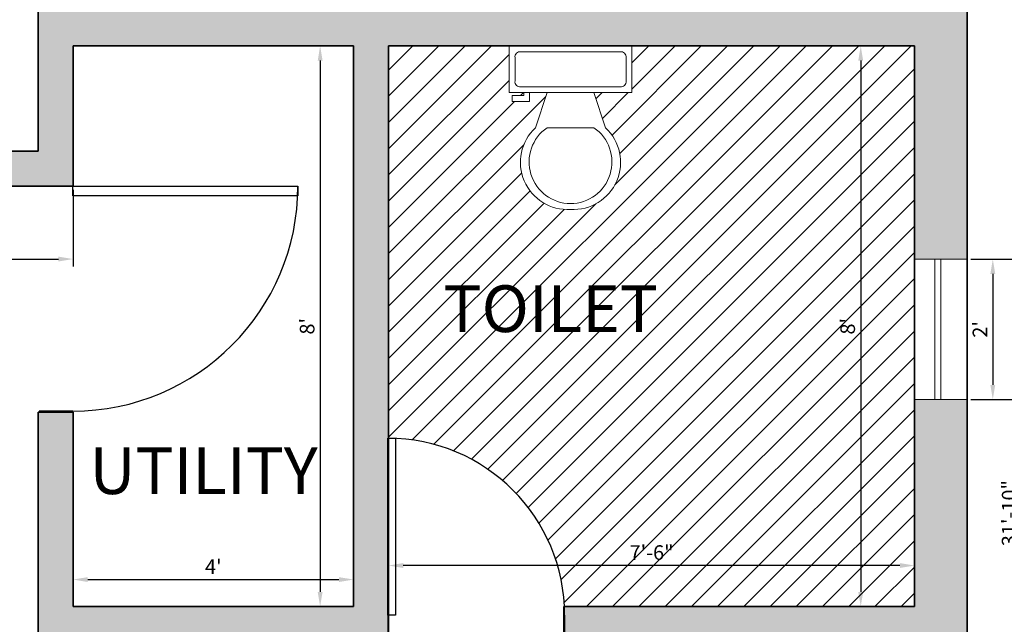
# Model space of a CAD drawing. Units: inches. Extents: x 2901 to 5923, y 918 to 2827.
# Tile 12 of 16: x 4730 to 4898, y 1420 to 1524. Entities that reach past the tile are written whole.
import ezdxf

# ---------------------------------------------------------------- set-up
doc = ezdxf.new("R2010")
doc.units = ezdxf.units.IN
for name, color, linetype, lineweight in [('A-ANNO-DIMS', 2, 'Continuous', 18), ('A-AREA-IDEN', 7, 'Continuous', 25), ('A-FLOR-FIXT', 9, 'Continuous', 18), ('A-FLOR-PATT', 252, 'Continuous', 13), ('A-GLAZ', 4, 'Continuous', 18), ('A-WALL-PATT', 7, 'Continuous', 13), ('doors', 240, 'Continuous', 25), ('walls', 7, 'Continuous', 35)]:
    doc.layers.add(name, color=color, linetype=linetype, lineweight=lineweight)
doc.styles.get("Standard").update_dxf_attribs({"font": 'arial.ttf'})
doc.dimstyles.new('Copy of ISO-25', dxfattribs={"dimtxt": 2.5, "dimasz": 2.5, "dimexe": 1.25, "dimexo": 0.625, "dimtad": 1, "dimdec": 1, "dimlunit": 4, "dimtxsty": 'Standard', "dimcen": 2.5, "dimadec": 0, "dimazin": 0, "dimtfac": 1, "dimtdec": 1, "dimtmove": 0, "dimatfit": 3, "dimfxl": 1, "dimarcsym": 0})

# ---------------------------------------------------------------- blocks, each defined once
blk = doc.blocks.new('*U4')
for p, q in [((-40, 0), (-40, 6)), ((0, 0), (0, 6))]:
    blk.add_line(p, q)
blk.add_lwpolyline([(0, 0), (0, -40), (-1.75, -40), (-1.75, 0)], close=True)
blk.add_arc((0, 0), 40, 180, 270)
blk = doc.blocks.new('*U2')
for p, q in [((0, 0), (0, -6)), ((40, 0), (40, -6))]:
    blk.add_line(p, q)
blk.add_lwpolyline([(0, 0), (0, 40), (1.75, 40), (1.75, 0)], close=True)
blk.add_arc((0, 0), 40, 0, 90)
blk = doc.blocks.new('*U20')
for p, q in [((241.3, -152.4), (241.3, -50.8)), ((-203.2, -215.9), (-203.2, -203.2)), ((-177.8, -203.2), (-177.8, -241.3)), ((-101.6, -203.2), (-152.4, -355.6)), ((101.6, -203.2), (152.4, -355.6)), ((-254, -215.9), (-203.2, -215.9)), ((-254, -241.3), (-254, -215.9)), ((-177.8, -241.3), (-254, -241.3)), ((101.6, -355.6), (-101.6, -355.6))]:
    blk.add_line(p, q)
blk.add_lwpolyline([(266.7, -203.2), (266.7, 0), (-266.7, 0), (-266.7, -203.2)], close=True)
for points in [[(215.9, -25.4), (-215.9, -25.4)], [(-241.3, -50.8), (-241.3, -152.4)], [(-215.9, -177.8), (215.9, -177.8)]]:
    blk.add_lwpolyline(points)
for centre, radius, start, end in [((-219.075, -47.625), 22.45064, 81.8699, 188.1301), ((219.075, -47.625), 22.45064, 351.8699, 98.1301), ((-219.075, -155.575), 22.45064, 171.869898, 278.1301), ((219.075, -155.575), 22.45064, 261.8699, 8.1301), ((-12.12088, -505.93752), 205.61935, 133.01722, 273.38), ((0.94996, -504.77674), 181.02486, 124.50543, 269.7), ((-0.94742, -504.77674), 181.02486, 270.3, 55.4946), ((12.12342, -505.93752), 205.61935, 266.62, 46.9828)]:
    blk.add_arc(centre, radius, start, end)
blk = doc.blocks.new('*D35')
at = {"layer": 'A-ANNO-DIMS', "color": 0, "lineweight": -2, "transparency": 16777216}
for p, q in [((4892.69, 1630.4), (4902.74, 1630.4)), ((4901.49, 1250.9), (4901.49, 1627.9)), ((4892.69, 1248.4), (4902.74, 1248.4))]:
    blk.add_line(p, q, dxfattribs=at)
at = {"layer": 'A-ANNO-DIMS', "color": 0, "transparency": 16777216}
for points in [[(4901.07, 1627.9), (4901.91, 1627.9), (4901.49, 1630.4)], [(4901.07, 1250.9), (4901.91, 1250.9), (4901.49, 1248.4)]]:
    blk.add_solid(points, dxfattribs=at)
at = {"layer": 'Defpoints', "color": 0, "transparency": 16777216}
for p in [(4892.07, 1630.4), (4901.49, 1630.4), (4892.07, 1248.4)]:
    blk.add_point(p, dxfattribs=at)
at = {"layer": 'A-ANNO-DIMS', "color": 0, "transparency": 16777216, "insert": (4899.59, 1439.4), "char_height": 2.5, "attachment_point": 5, "rotation": 90}
blk.add_mtext('31\'-10"', dxfattribs=at)
blk = doc.blocks.new('*D44')
at = {"layer": 'A-ANNO-DIMS', "color": 0, "lineweight": -2, "transparency": 16777216}
for p, q in [((4882.44, 1519.4), (4872.62, 1519.4)), ((4873.87, 1516.9), (4873.87, 1425.9)), ((4882.44, 1423.4), (4872.62, 1423.4))]:
    blk.add_line(p, q, dxfattribs=at)
at = {"layer": 'A-ANNO-DIMS', "color": 0, "transparency": 16777216}
for points in [[(4873.45, 1516.9), (4874.28, 1516.9), (4873.87, 1519.4)], [(4873.45, 1425.9), (4874.28, 1425.9), (4873.87, 1423.4)]]:
    blk.add_solid(points, dxfattribs=at)
at = {"layer": 'Defpoints', "color": 0, "transparency": 16777216}
for p in [(4883.07, 1519.4), (4873.87, 1423.4), (4883.07, 1423.4)]:
    blk.add_point(p, dxfattribs=at)
at = {"layer": 'A-ANNO-DIMS', "color": 0, "transparency": 16777216, "insert": (4871.96, 1471.4), "char_height": 2.5, "attachment_point": 5, "rotation": 90}
blk.add_mtext("8'", dxfattribs=at)
blk = doc.blocks.new('*D45')
at = {"layer": 'A-ANNO-DIMS', "color": 0, "lineweight": -2, "transparency": 16777216}
for p, q in [((4793.07, 1424.02), (4793.07, 1431.68)), ((4883.07, 1424.02), (4883.07, 1431.68)), ((4880.57, 1430.43), (4795.57, 1430.43))]:
    blk.add_line(p, q, dxfattribs=at)
at = {"layer": 'A-ANNO-DIMS', "color": 0, "transparency": 16777216}
for points in [[(4795.57, 1430.85), (4795.57, 1430.01), (4793.07, 1430.43)], [(4880.57, 1430.85), (4880.57, 1430.01), (4883.07, 1430.43)]]:
    blk.add_solid(points, dxfattribs=at)
at = {"layer": 'Defpoints', "color": 0, "transparency": 16777216}
for p in [(4793.07, 1430.43), (4793.07, 1423.4), (4883.07, 1423.4)]:
    blk.add_point(p, dxfattribs=at)
at = {"layer": 'A-ANNO-DIMS', "color": 0, "transparency": 16777216, "insert": (4838.07, 1432.33), "char_height": 2.5, "attachment_point": 5}
blk.add_mtext('7\'-6"', dxfattribs=at)
blk = doc.blocks.new('*D46')
at = {"layer": 'A-ANNO-DIMS', "color": 0, "lineweight": -2, "transparency": 16777216}
for p, q in [((4739.07, 1424.02), (4739.07, 1429.28)), ((4787.07, 1424.02), (4787.07, 1429.28)), ((4741.57, 1428.03), (4784.57, 1428.03))]:
    blk.add_line(p, q, dxfattribs=at)
at = {"layer": 'A-ANNO-DIMS', "color": 0, "transparency": 16777216}
for points in [[(4741.57, 1428.44), (4741.57, 1427.61), (4739.07, 1428.03)], [(4784.57, 1428.44), (4784.57, 1427.61), (4787.07, 1428.03)]]:
    blk.add_solid(points, dxfattribs=at)
at = {"layer": 'Defpoints', "color": 0, "transparency": 16777216}
for p in [(4787.07, 1428.03), (4739.07, 1423.4), (4787.07, 1423.4)]:
    blk.add_point(p, dxfattribs=at)
at = {"layer": 'A-ANNO-DIMS', "color": 0, "transparency": 16777216, "insert": (4763.07, 1429.9), "char_height": 2.5, "attachment_point": 5}
blk.add_mtext("4'", dxfattribs=at)
blk = doc.blocks.new('*D47')
at = {"layer": 'A-ANNO-DIMS', "color": 0, "lineweight": -2, "transparency": 16777216}
for p, q in [((4786.44, 1519.4), (4780.1, 1519.4)), ((4781.35, 1516.9), (4781.35, 1425.9)), ((4786.44, 1423.4), (4780.1, 1423.4))]:
    blk.add_line(p, q, dxfattribs=at)
at = {"layer": 'A-ANNO-DIMS', "color": 0, "transparency": 16777216}
for points in [[(4780.94, 1516.9), (4781.77, 1516.9), (4781.35, 1519.4)], [(4780.94, 1425.9), (4781.77, 1425.9), (4781.35, 1423.4)]]:
    blk.add_solid(points, dxfattribs=at)
at = {"layer": 'Defpoints', "color": 0, "transparency": 16777216}
for p in [(4787.07, 1519.4), (4781.35, 1423.4), (4787.07, 1423.4)]:
    blk.add_point(p, dxfattribs=at)
at = {"layer": 'A-ANNO-DIMS', "color": 0, "transparency": 16777216, "insert": (4779.45, 1471.4), "char_height": 2.5, "attachment_point": 5, "rotation": 90}
blk.add_mtext("8'", dxfattribs=at)
blk = doc.blocks.new('*D56')
at = {"layer": 'A-ANNO-DIMS', "color": 0, "lineweight": -2, "transparency": 16777216}
for p, q in [((4589.07, 1494.77), (4589.07, 1481.66)), ((4739.07, 1494.77), (4739.07, 1481.66)), ((4591.57, 1482.91), (4736.57, 1482.91))]:
    blk.add_line(p, q, dxfattribs=at)
at = {"layer": 'A-ANNO-DIMS', "color": 0, "transparency": 16777216}
for points in [[(4591.57, 1483.32), (4591.57, 1482.49), (4589.07, 1482.91)], [(4736.57, 1483.32), (4736.57, 1482.49), (4739.07, 1482.91)]]:
    blk.add_solid(points, dxfattribs=at)
at = {"layer": 'Defpoints', "color": 0, "transparency": 16777216}
for p in [(4589.07, 1495.4), (4739.07, 1495.4), (4739.07, 1482.91)]:
    blk.add_point(p, dxfattribs=at)
at = {"layer": 'A-ANNO-DIMS', "color": 0, "transparency": 16777216, "insert": (4664.07, 1484.81), "char_height": 2.5, "attachment_point": 5}
blk.add_mtext('12\'-6"', dxfattribs=at)
blk = doc.blocks.new('*D69')
at = {"layer": 'A-ANNO-DIMS', "color": 0, "lineweight": -2, "transparency": 16777216}
for p, q in [((4892.69, 1482.87), (4897.72, 1482.87)), ((4896.47, 1480.37), (4896.47, 1461.37)), ((4892.69, 1458.87), (4897.72, 1458.87))]:
    blk.add_line(p, q, dxfattribs=at)
at = {"layer": 'A-ANNO-DIMS', "color": 0, "transparency": 16777216}
for points in [[(4896.05, 1480.37), (4896.89, 1480.37), (4896.47, 1482.87)], [(4896.05, 1461.37), (4896.89, 1461.37), (4896.47, 1458.87)]]:
    blk.add_solid(points, dxfattribs=at)
at = {"layer": 'Defpoints', "color": 0, "transparency": 16777216}
for p in [(4892.07, 1482.87), (4892.07, 1458.87), (4896.47, 1458.87)]:
    blk.add_point(p, dxfattribs=at)
at = {"layer": 'A-ANNO-DIMS', "color": 0, "transparency": 16777216, "insert": (4894.59, 1470.87), "char_height": 2.5, "attachment_point": 5, "rotation": 90}
blk.add_mtext("2'", dxfattribs=at)
blk = doc.blocks.new('*D89')
at = {"layer": 'A-ANNO-DIMS', "color": 0, "lineweight": -2, "transparency": 16777216}
for p, q in [((4892.69, 1630.4), (5055.73, 1630.4)), ((5054.48, 989.9), (5054.48, 1627.9)), ((4709.69, 987.4), (5055.73, 987.4))]:
    blk.add_line(p, q, dxfattribs=at)
at = {"layer": 'A-ANNO-DIMS', "color": 0, "transparency": 16777216}
for points in [[(5054.06, 1627.9), (5054.9, 1627.9), (5054.48, 1630.4)], [(5054.06, 989.9), (5054.9, 989.9), (5054.48, 987.4)]]:
    blk.add_solid(points, dxfattribs=at)
at = {"layer": 'Defpoints', "color": 0, "transparency": 16777216}
for p in [(4892.07, 1630.4), (5054.48, 1630.4), (4709.07, 987.4)]:
    blk.add_point(p, dxfattribs=at)
at = {"layer": 'A-ANNO-DIMS', "color": 0, "transparency": 16777216, "insert": (5052.58, 1308.9), "char_height": 2.5, "attachment_point": 5, "rotation": 90}
blk.add_mtext('53\'-7"', dxfattribs=at)
blk = doc.blocks.new('*D96')
at = {"layer": 'A-ANNO-DIMS', "color": 0, "lineweight": -2, "transparency": 16777216}
for p, q in [((4892.69, 1630.4), (5055.73, 1630.4)), ((5054.48, 1627.9), (5054.48, 1485.37)), ((4892.69, 1482.87), (5055.73, 1482.87))]:
    blk.add_line(p, q, dxfattribs=at)
at = {"layer": 'A-ANNO-DIMS', "color": 0, "transparency": 16777216}
for points in [[(5054.06, 1627.9), (5054.9, 1627.9), (5054.48, 1630.4)], [(5054.06, 1485.37), (5054.9, 1485.37), (5054.48, 1482.87)]]:
    blk.add_solid(points, dxfattribs=at)
at = {"layer": 'Defpoints', "color": 0, "transparency": 16777216}
for p in [(4892.07, 1630.4), (4892.07, 1482.87), (5054.48, 1482.87)]:
    blk.add_point(p, dxfattribs=at)
at = {"layer": 'A-ANNO-DIMS', "color": 0, "transparency": 16777216, "insert": (5052.56, 1556.63), "char_height": 2.5, "attachment_point": 5, "rotation": 90}
blk.add_mtext('12\'-3 1/2"', dxfattribs=at)
blk = doc.blocks.new('*D97')
at = {"layer": 'A-ANNO-DIMS', "color": 0, "lineweight": -2, "transparency": 16777216}
for p, q in [((4892.69, 1458.87), (5055.73, 1458.87)), ((5054.48, 1456.37), (5054.48, 1365.81)), ((4892.69, 1363.31), (5055.73, 1363.31))]:
    blk.add_line(p, q, dxfattribs=at)
at = {"layer": 'A-ANNO-DIMS', "color": 0, "transparency": 16777216}
for points in [[(5054.06, 1456.37), (5054.9, 1456.37), (5054.48, 1458.87)], [(5054.06, 1365.81), (5054.9, 1365.81), (5054.48, 1363.31)]]:
    blk.add_solid(points, dxfattribs=at)
at = {"layer": 'Defpoints', "color": 0, "transparency": 16777216}
for p in [(4892.07, 1458.87), (4892.07, 1363.31), (5054.48, 1363.31)]:
    blk.add_point(p, dxfattribs=at)
at = {"layer": 'A-ANNO-DIMS', "color": 0, "transparency": 16777216, "insert": (5052.56, 1411.09), "char_height": 2.5, "attachment_point": 5, "rotation": 90}
blk.add_mtext('7\'-11 1/2"', dxfattribs=at)

msp = doc.modelspace()

# ---------------------------------------------------------------- hatches: boundary and pattern name
at = {"layer": 'A-FLOR-PATT'}
h = msp.add_hatch(dxfattribs=at)
h.set_pattern_fill('ANSI32', color=256)
h.paths.add_polyline_path([(4883.07, 1621.4), (4739.07, 1621.4), (4739.07, 1564.39, -0.396616), (4774.43, 1529.97), (4774.46, 1529.97), (4774.46, 1528.4), (4883.07, 1528.4)])
h.paths.add_polyline_path([(4733.07, 1143.4), (4685.07, 1143.4), (4685.07, 1147.03), (4684.01, 1147.03), (4684.01, 1171.22, 0.413071), (4660.87, 1146.06, 0.412532), (4638.11, 1170.77), (4638.11, 1146.97), (4637.07, 1143.4), (4589.07, 1143.4), (4589.07, 1029.4), (4733.07, 1029.4)])
h.paths.add_polyline_path([(4620.35, 1086.26, -0.333335), (4622.56, 1084.04), (4622.56, 1084.04), (4712.62, 1084.04, -0.333335), (4714.84, 1086.26), (4718.53, 1086.26, -0.376086), (4721.48, 1084.04), (4721.48, 1062.64), (4721.48, 1041.23, -0.333387), (4718.96, 1039.01), (4714.84, 1039.01, -0.333335), (4712.62, 1041.23), (4712.62, 1041.23), (4622.56, 1041.23, -0.333335), (4620.35, 1039.01), (4616.66, 1039.01, -0.376086), (4613.71, 1041.23), (4613.71, 1062.63), (4613.71, 1084.04, -0.333387), (4616.23, 1086.26)], flags=16)
h.paths.add_polyline_path([(4638.8, 1084.04), (4643.23, 1078.14), (4678.67, 1078.14), (4687.53, 1084.04), (4687.53, 1071.49), (4718.53, 1067.06), (4718.53, 1062.64), (4718.53, 1058.21), (4687.53, 1053.78), (4687.53, 1041.23), (4678.67, 1047.13), (4643.23, 1047.13), (4638.8, 1041.23), (4638.8, 1062.63)], flags=0)
h = msp.add_hatch(dxfattribs=at)
h.set_pattern_fill('ANSI31', color=256)
h.paths.add_polyline_path([(4883.07, 1519.4), (4834.7, 1519.4), (4834.7, 1511.4), (4828.2, 1511.4), (4830.2, 1505.4, -0.702571), (4824.2, 1491.4, -0.702562), (4818.2, 1505.4), (4820.2, 1511.4), (4817.2, 1511.4), (4817.2, 1509.9), (4814.2, 1509.9), (4814.2, 1510.9), (4816.2, 1510.9), (4816.2, 1511.4), (4813.7, 1511.4), (4813.7, 1519.4), (4793.07, 1519.4), (4793.07, 1452.23), (4794.23, 1452.23), (4794.23, 1452.2, -0.387553), (4823.16, 1423.4), (4883.07, 1423.4)])
at = {"layer": 'A-WALL-PATT'}
h = msp.add_hatch(color=256, dxfattribs=at)
h.dxf.hatch_style = 1
h.paths.add_polyline_path([(4439.07, 1447.4), (4583.07, 1447.4), (4583.07, 1340.4), (4589.07, 1340.4), (4589.07, 1453.4), (4589.07, 1455.39), (4583.07, 1455.39), (4583.07, 1453.4), (4439.07, 1453.4), (4439.07, 1501.84), (4430.07, 1501.84), (4430.07, 1399.4), (4439.07, 1399.4)])
h.paths.add_polyline_path([(4439.07, 1621.4), (4487.07, 1621.4), (4487.07, 1630.4), (4430.07, 1630.4), (4430.07, 1561.84), (4439.07, 1561.84)])
h.paths.add_polyline_path([(4630.61, 1630.4), (4535.07, 1630.4), (4535.07, 1621.4), (4583.07, 1621.4), (4583.07, 1495.4), (4589.07, 1495.4), (4637.07, 1495.4), (4637.07, 1501.4), (4589.07, 1501.4), (4589.07, 1621.4), (4630.61, 1621.4)])
h.paths.add_polyline_path([(4892.07, 1630.4), (4690.61, 1630.4), (4690.61, 1621.4), (4733.07, 1621.4), (4733.07, 1564.4), (4739.07, 1564.4), (4739.07, 1621.4), (4883.07, 1621.4), (4883.07, 1528.4), (4739.07, 1528.4), (4733.07, 1528.4), (4733.07, 1501.4), (4685.07, 1501.4), (4685.07, 1495.4), (4739.07, 1495.4), (4739.07, 1519.4), (4787.07, 1519.4), (4787.07, 1423.4), (4739.07, 1423.4), (4739.07, 1456.67), (4733.07, 1456.67), (4733.07, 1340.4), (4739.07, 1340.4), (4739.07, 1417.4), (4787.07, 1417.4), (4793.07, 1417.4), (4793.07, 1423.4), (4793.07, 1519.4), (4883.07, 1519.4), (4883.07, 1482.87), (4892.07, 1482.87)])
h.paths.add_polyline_path([(4892.07, 1458.87), (4883.07, 1458.87), (4883.07, 1423.4), (4823.07, 1423.4), (4823.07, 1417.4), (4883.07, 1417.4), (4883.07, 1363.31), (4892.07, 1363.31)], flags=17)
h.paths.add_polyline_path([(4892.07, 1303.31), (4883.07, 1303.31), (4883.07, 1255.4), (4739.07, 1255.4), (4739.07, 1304.4), (4733.07, 1304.4), (4733.07, 1303.4), (4733.07, 1297.4), (4733.07, 1255.4), (4733.07, 1248.4), (4811.07, 1248.4), (4811.07, 1212.16), (4820.07, 1212.16), (4820.07, 1248.4), (4892.07, 1248.4)])
h.paths.add_polyline_path([(4820.07, 1182.16), (4811.07, 1182.16), (4811.07, 1152.4), (4685.07, 1152.4), (4685.07, 1147.03), (4685.07, 1143.4), (4733.07, 1143.4), (4811.07, 1143.4), (4814.07, 1143.4), (4820.07, 1143.4)])
h.paths.add_polyline_path([(4637.07, 1152.4), (4589.07, 1152.4), (4589.07, 1153.4), (4583.86, 1153.4), (4583.07, 1153.4), (4583.07, 1152.4), (4511.07, 1152.4), (4511.07, 1182.16), (4502.07, 1182.16), (4502.07, 1143.4), (4568.07, 1143.4), (4583.07, 1143.4), (4583.07, 1023.4), (4739.07, 1023.4), (4739.07, 1143.4), (4733.07, 1143.4), (4733.07, 1029.4), (4589.07, 1029.4), (4589.07, 1143.4), (4637.07, 1143.4), (4637.07, 1146.97)])
h.paths.add_polyline_path([(4511.07, 1246.4), (4583.07, 1246.4), (4583.07, 1188.4), (4589.07, 1188.4), (4589.07, 1246.4), (4589.07, 1248.4), (4589.07, 1255.4), (4589.07, 1297.4), (4697.07, 1297.4), (4697.07, 1303.4), (4589.07, 1303.4), (4589.07, 1304.4), (4583.07, 1304.4), (4583.07, 1255.4), (4439.07, 1255.4), (4439.07, 1261.4), (4439.07, 1351.4), (4430.07, 1351.4), (4430.07, 1252.4), (4430.07, 1246.4), (4439.07, 1246.4), (4487.07, 1246.4), (4502.07, 1246.4), (4502.07, 1212.16), (4511.07, 1212.16)])

# ---------------------------------------------------------------- linework, layer by layer
at = {"layer": 'A-GLAZ'}
for p, q in [((4883.07, 1482.87), (4892.07, 1482.87)), ((4886.57, 1482.87), (4886.57, 1458.87)), ((4887.57, 1482.87), (4887.57, 1458.87)), ((4892.07, 1482.87), (4892.07, 1458.87)), ((4892.07, 1458.87), (4883.07, 1458.87))]:
    msp.add_line(p, q, dxfattribs=at)
at = {"layer": 'walls'}
for p, q in [((4892.07, 1630.4), (4892.07, 1248.4)), ((4733.07, 1528.4), (4733.07, 1501.4)), ((4739.07, 1519.4), (4787.07, 1519.4)), ((4787.07, 1519.4), (4739.07, 1519.4)), ((4739.07, 1519.4), (4739.07, 1495.4)), ((4787.07, 1519.4), (4787.07, 1423.4)), ((4883.07, 1519.4), (4793.07, 1519.4)), ((4883.07, 1519.4), (4793.07, 1519.4)), ((4793.07, 1519.4), (4793.07, 1423.4)), ((4793.07, 1519.4), (4872.17, 1519.4)), ((4883.07, 1519.4), (4883.07, 1423.4)), ((4733.07, 1501.4), (4685.07, 1501.4)), ((4739.07, 1495.4), (4685.07, 1495.4)), ((4739.07, 1456.67), (4733.07, 1456.67)), ((4733.07, 1456.67), (4733.07, 1340.4)), ((4739.07, 1423.4), (4739.07, 1456.67)), ((4739.07, 1423.4), (4787.07, 1423.4)), ((4793.07, 1423.4), (4793.07, 1417.4)), ((4823.07, 1423.4), (4883.07, 1423.4)), ((4823.07, 1423.4), (4823.07, 1417.4))]:
    msp.add_line(p, q, dxfattribs=at)

# ---------------------------------------------------------------- block references
at = {"layer": 'A-FLOR-FIXT', "xscale": 0.0393700787401575, "yscale": 0.0393700787401575, "zscale": 0.0393700787401575}
msp.add_blockref('*U20', (4824.2, 1519.4), dxfattribs=at)
at = {"layer": 'doors', "xscale": 0.9632045105573293, "yscale": 0.9632045105573293, "zscale": 0.9632045105573293, "rotation": 90}
msp.add_blockref('*U4', (4739.02, 1495.4), dxfattribs=at)
at = {"layer": 'doors', "xscale": 0.7572280359034433, "yscale": 0.7572280359034433, "zscale": 0.7572280359034433}
msp.add_blockref('*U2', (4792.91, 1421.94), dxfattribs=at)

# ---------------------------------------------------------------- texts
at = {"layer": 'A-AREA-IDEN'}
for s, p in [('TOILET', (4802.45, 1470.41)), ('UTILITY', (4741.87, 1442.67))]:
    msp.add_text(s, height=8, dxfattribs=at).set_placement(p)

# ---------------------------------------------------------------- dimensions: what is measured, and where the dimension line sits
at = {"layer": 'A-ANNO-DIMS'}
for base, p1, p2, override, picture, middle in [((5054.48, 1630.4), (4709.07, 987.4), (4892.07, 1630.4), {"dimdec": 1, "dimlfac": 1, "dimrnd": 0, "dimzin": 1, "dimdsep": 46, "dimlunit": 4, "dimfrac": 2}, '*D89', (5052.58, 1308.9)), ((4901.49, 1630.4), (4892.07, 1248.4), (4892.07, 1630.4), {"dimclrd": 0, "dimclre": 0, "dimclrt": 0}, '*D35', (4899.59, 1439.4)), ((5054.48, 1482.87), (4892.07, 1630.4), (4892.07, 1482.87), {"dimdec": 1, "dimlfac": 1, "dimrnd": 0, "dimzin": 1, "dimdsep": 46, "dimlunit": 4, "dimfrac": 2}, '*D96', (5052.56, 1556.63)), ((4781.35, 1423.4), (4787.07, 1519.4), (4787.07, 1423.4), {"dimclrd": 0, "dimclre": 0, "dimclrt": 0}, '*D47', (4779.45, 1471.4)), ((4873.87, 1423.4), (4883.07, 1519.4), (4883.07, 1423.4), {"dimclrd": 0, "dimclre": 0, "dimclrt": 0}, '*D44', (4871.96, 1471.4)), ((4896.47, 1458.87), (4892.07, 1482.87), (4892.07, 1458.87), {"dimclrd": 0, "dimclre": 0, "dimclrt": 0}, '*D69', (4894.59, 1470.87)), ((5054.48, 1363.31), (4892.07, 1458.87), (4892.07, 1363.31), {"dimdec": 1, "dimlfac": 1, "dimrnd": 0, "dimzin": 1, "dimdsep": 46, "dimlunit": 4, "dimfrac": 2}, '*D97', (5052.56, 1411.09))]:
    dim = msp.add_linear_dim(base=base, p1=p1, p2=p2, angle=90, dimstyle='Copy of ISO-25', override=override, dxfattribs=at)
    dim.commit()
    dim.dimension.update_dxf_attribs({"geometry": picture, "text_midpoint": middle})
for base, p1, p2, picture, middle in [((4739.07, 1482.91), (4589.07, 1495.4), (4739.07, 1495.4), '*D56', (4664.07, 1484.81)), ((4793.07, 1430.43), (4883.07, 1423.4), (4793.07, 1423.4), '*D45', (4838.07, 1432.33)), ((4787.07, 1428.03), (4739.07, 1423.4), (4787.07, 1423.4), '*D46', (4763.07, 1429.9))]:
    dim = msp.add_linear_dim(base=base, p1=p1, p2=p2, dimstyle='Copy of ISO-25', override={"dimclrd": 0, "dimclre": 0, "dimclrt": 0}, dxfattribs=at)
    dim.commit()
    dim.dimension.update_dxf_attribs({"geometry": picture, "text_midpoint": middle})

doc.saveas('drawing.dxf')
